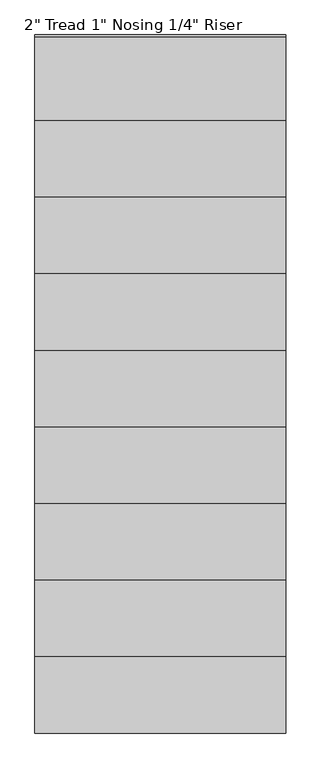
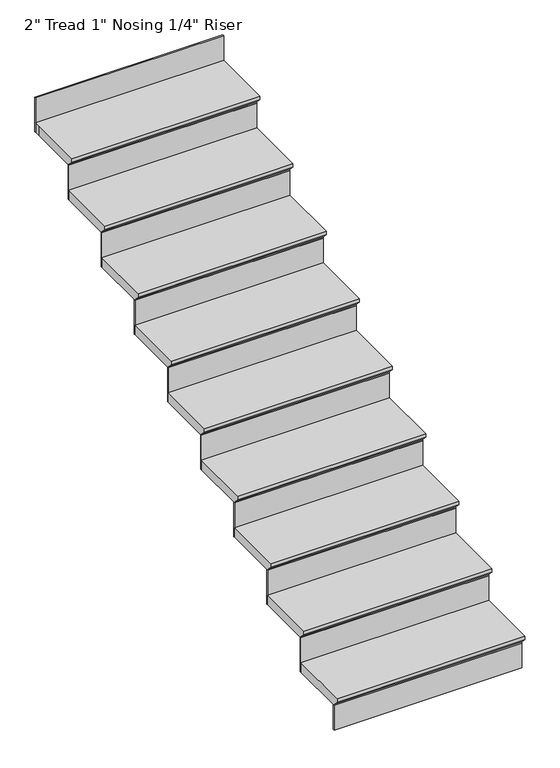
"""IFC4 building model written with IfcOpenShell, lengths in millimetres: stair flight geometry."""

from ifc_helpers import new_model, si_unit, origin, place, context, project, spatial, faceted_brep, source, transform, mapped, element, save


def stair_flight_52e4cb2b(model_context):
    return source(origin(), model_context, "Body", "Brep", [
        faceted_brep([(8378.8260838, -1689.0339187, 7169.15), (8378.8260838, -1689.0339187, 7188.2), (7464.4260838, -1689.0339187, 7188.2), (7464.4260838, -1689.0339187, 7169.15), (8378.8260838, -1663.6339187, 7143.75), (7464.4260838, -1663.6339187, 7143.75), (8378.8260838, -1384.2339187, 7188.2), (7464.4260838, -1384.2339187, 7188.2), (7464.4260838, -1663.6339187, 7137.4), (7464.4260838, -1384.2339187, 7137.4), (8378.8260838, -1384.2339187, 7137.4), (8378.8260838, -1663.6339187, 7137.4)], [[[0, 1, 2, 3]], [[4, 0, 3, 5]], [[2, 1, 6, 7]], [[8, 9, 10, 11]], [[2, 7, 9, 8, 5, 3]], [[8, 11, 4, 5]], [[6, 1, 0, 4, 11, 10]], [[7, 6, 10, 9]]]),
        faceted_brep([(8378.8260838, -1663.6339187, 7137.4), (8378.8260838, -1663.6339187, 7010.4), (8378.8260838, -1657.2839187, 7010.4), (8378.8260838, -1657.2839187, 7137.4), (7464.4260838, -1663.6339187, 7137.4), (7464.4260838, -1657.2839187, 7137.4), (7464.4260838, -1657.2839187, 7010.4), (7464.4260838, -1663.6339187, 7010.4)], [[[0, 1, 2, 3]], [[4, 5, 6, 7]], [[1, 0, 4, 7]], [[2, 1, 7, 6]], [[3, 2, 6, 5]], [[0, 3, 5, 4]]]),
        faceted_brep([(8378.8260838, -1384.2339187, 7315.2), (8378.8260838, -1384.2339187, 7137.4), (8378.8260838, -1377.8839187, 7137.4), (8378.8260838, -1377.8839187, 7315.2), (7464.4260838, -1384.2339187, 7315.2), (7464.4260838, -1377.8839187, 7315.2), (7464.4260838, -1377.8839187, 7137.4), (7464.4260838, -1384.2339187, 7137.4)], [[[0, 1, 2, 3]], [[4, 5, 6, 7]], [[1, 0, 4, 7]], [[2, 1, 7, 6]], [[3, 2, 6, 5]], [[0, 3, 5, 4]]]),
        faceted_brep([(7464.4260838, -1409.6339187, 7366.0), (8378.8260838, -1409.6339187, 7366.0), (8378.8260838, -1104.8339187, 7366.0), (7464.4260838, -1104.8339187, 7366.0), (7464.4260838, -1384.2339187, 7315.2), (7464.4260838, -1104.8339187, 7315.2), (8378.8260838, -1104.8339187, 7315.2), (8378.8260838, -1384.2339187, 7315.2), (7464.4260838, -1384.2339187, 7321.55), (7464.4260838, -1409.6339187, 7346.95), (8378.8260838, -1384.2339187, 7321.55), (8378.8260838, -1409.6339187, 7346.95)], [[[0, 1, 2, 3]], [[4, 5, 6, 7]], [[0, 3, 5, 4, 8, 9]], [[4, 7, 10, 8]], [[2, 1, 11, 10, 7, 6]], [[3, 2, 6, 5]], [[11, 1, 0, 9]], [[10, 11, 9, 8]]]),
        faceted_brep([(8378.8260838, -1104.8339187, 7493.0), (8378.8260838, -1104.8339187, 7315.2), (8378.8260838, -1098.4839187, 7315.2), (8378.8260838, -1098.4839187, 7493.0), (7464.4260838, -1104.8339187, 7493.0), (7464.4260838, -1098.4839187, 7493.0), (7464.4260838, -1098.4839187, 7315.2), (7464.4260838, -1104.8339187, 7315.2)], [[[0, 1, 2, 3]], [[4, 5, 6, 7]], [[1, 0, 4, 7]], [[2, 1, 7, 6]], [[3, 2, 6, 5]], [[0, 3, 5, 4]]]),
        faceted_brep([(7464.4260838, -1130.2339187, 7543.8), (8378.8260838, -1130.2339187, 7543.8), (8378.8260838, -825.4339187, 7543.8), (7464.4260838, -825.4339187, 7543.8), (7464.4260838, -1104.8339187, 7493.0), (7464.4260838, -825.4339187, 7493.0), (8378.8260838, -825.4339187, 7493.0), (8378.8260838, -1104.8339187, 7493.0), (7464.4260838, -1104.8339187, 7499.35), (7464.4260838, -1130.2339187, 7524.75), (8378.8260838, -1104.8339187, 7499.35), (8378.8260838, -1130.2339187, 7524.75)], [[[0, 1, 2, 3]], [[4, 5, 6, 7]], [[0, 3, 5, 4, 8, 9]], [[4, 7, 10, 8]], [[2, 1, 11, 10, 7, 6]], [[3, 2, 6, 5]], [[11, 1, 0, 9]], [[10, 11, 9, 8]]]),
        faceted_brep([(8378.8260838, -825.4339187, 7670.8), (8378.8260838, -825.4339187, 7493.0), (8378.8260838, -819.0839187, 7493.0), (8378.8260838, -819.0839187, 7670.8), (7464.4260838, -825.4339187, 7670.8), (7464.4260838, -819.0839187, 7670.8), (7464.4260838, -819.0839187, 7493.0), (7464.4260838, -825.4339187, 7493.0)], [[[0, 1, 2, 3]], [[4, 5, 6, 7]], [[1, 0, 4, 7]], [[2, 1, 7, 6]], [[3, 2, 6, 5]], [[0, 3, 5, 4]]]),
        faceted_brep([(7464.4260838, -850.8339187, 7721.6), (8378.8260838, -850.8339187, 7721.6), (8378.8260838, -546.0339187, 7721.6), (7464.4260838, -546.0339187, 7721.6), (7464.4260838, -825.4339187, 7670.8), (7464.4260838, -546.0339187, 7670.8), (8378.8260838, -546.0339187, 7670.8), (8378.8260838, -825.4339187, 7670.8), (7464.4260838, -825.4339187, 7677.15), (7464.4260838, -850.8339187, 7702.55), (8378.8260838, -825.4339187, 7677.15), (8378.8260838, -850.8339187, 7702.55)], [[[0, 1, 2, 3]], [[4, 5, 6, 7]], [[0, 3, 5, 4, 8, 9]], [[4, 7, 10, 8]], [[2, 1, 11, 10, 7, 6]], [[3, 2, 6, 5]], [[11, 1, 0, 9]], [[10, 11, 9, 8]]]),
        faceted_brep([(8378.8260838, -546.0339187, 7848.6), (8378.8260838, -546.0339187, 7670.8), (8378.8260838, -539.6839187, 7670.8), (8378.8260838, -539.6839187, 7848.6), (7464.4260838, -546.0339187, 7848.6), (7464.4260838, -539.6839187, 7848.6), (7464.4260838, -539.6839187, 7670.8), (7464.4260838, -546.0339187, 7670.8)], [[[0, 1, 2, 3]], [[4, 5, 6, 7]], [[1, 0, 4, 7]], [[2, 1, 7, 6]], [[3, 2, 6, 5]], [[0, 3, 5, 4]]]),
        faceted_brep([(7464.4260838, -571.4339187, 7899.4), (8378.8260838, -571.4339187, 7899.4), (8378.8260838, -266.6339187, 7899.4), (7464.4260838, -266.6339187, 7899.4), (7464.4260838, -546.0339187, 7848.6), (7464.4260838, -266.6339187, 7848.6), (8378.8260838, -266.6339187, 7848.6), (8378.8260838, -546.0339187, 7848.6), (7464.4260838, -546.0339187, 7854.95), (7464.4260838, -571.4339187, 7880.35), (8378.8260838, -546.0339187, 7854.95), (8378.8260838, -571.4339187, 7880.35)], [[[0, 1, 2, 3]], [[4, 5, 6, 7]], [[0, 3, 5, 4, 8, 9]], [[4, 7, 10, 8]], [[2, 1, 11, 10, 7, 6]], [[3, 2, 6, 5]], [[11, 1, 0, 9]], [[10, 11, 9, 8]]]),
        faceted_brep([(8378.8260838, -266.6339187, 8026.4), (8378.8260838, -266.6339187, 7848.6), (8378.8260838, -260.2839187, 7848.6), (8378.8260838, -260.2839187, 8026.4), (7464.4260838, -266.6339187, 8026.4), (7464.4260838, -260.2839187, 8026.4), (7464.4260838, -260.2839187, 7848.6), (7464.4260838, -266.6339187, 7848.6)], [[[0, 1, 2, 3]], [[4, 5, 6, 7]], [[1, 0, 4, 7]], [[2, 1, 7, 6]], [[3, 2, 6, 5]], [[0, 3, 5, 4]]]),
        faceted_brep([(7464.4260838, -292.0339187, 8077.2), (8378.8260838, -292.0339187, 8077.2), (8378.8260838, 12.7660813, 8077.2), (7464.4260838, 12.7660813, 8077.2), (7464.4260838, -266.6339187, 8026.4), (7464.4260838, 12.7660813, 8026.4), (8378.8260838, 12.7660813, 8026.4), (8378.8260838, -266.6339187, 8026.4), (7464.4260838, -266.6339187, 8032.75), (7464.4260838, -292.0339187, 8058.15), (8378.8260838, -266.6339187, 8032.75), (8378.8260838, -292.0339187, 8058.15)], [[[0, 1, 2, 3]], [[4, 5, 6, 7]], [[0, 3, 5, 4, 8, 9]], [[4, 7, 10, 8]], [[2, 1, 11, 10, 7, 6]], [[3, 2, 6, 5]], [[11, 1, 0, 9]], [[10, 11, 9, 8]]]),
        faceted_brep([(8378.8260838, 12.7660813, 8204.2), (8378.8260838, 12.7660813, 8026.4), (8378.8260838, 19.1160813, 8026.4), (8378.8260838, 19.1160813, 8204.2), (7464.4260838, 12.7660813, 8204.2), (7464.4260838, 19.1160813, 8204.2), (7464.4260838, 19.1160813, 8026.4), (7464.4260838, 12.7660813, 8026.4)], [[[0, 1, 2, 3]], [[4, 5, 6, 7]], [[1, 0, 4, 7]], [[2, 1, 7, 6]], [[3, 2, 6, 5]], [[0, 3, 5, 4]]]),
        faceted_brep([(7464.4260838, -12.6339187, 8255.0), (8378.8260838, -12.6339187, 8255.0), (8378.8260838, 292.1660813, 8255.0), (7464.4260838, 292.1660813, 8255.0), (7464.4260838, 12.7660813, 8204.2), (7464.4260838, 292.1660813, 8204.2), (8378.8260838, 292.1660813, 8204.2), (8378.8260838, 12.7660813, 8204.2), (7464.4260838, 12.7660813, 8210.55), (7464.4260838, -12.6339187, 8235.95), (8378.8260838, 12.7660813, 8210.55), (8378.8260838, -12.6339187, 8235.95)], [[[0, 1, 2, 3]], [[4, 5, 6, 7]], [[0, 3, 5, 4, 8, 9]], [[4, 7, 10, 8]], [[2, 1, 11, 10, 7, 6]], [[3, 2, 6, 5]], [[11, 1, 0, 9]], [[10, 11, 9, 8]]]),
        faceted_brep([(8378.8260838, 292.1660813, 8382.0), (8378.8260838, 292.1660813, 8204.2), (8378.8260838, 298.5160813, 8204.2), (8378.8260838, 298.5160813, 8382.0), (7464.4260838, 292.1660813, 8382.0), (7464.4260838, 298.5160813, 8382.0), (7464.4260838, 298.5160813, 8204.2), (7464.4260838, 292.1660813, 8204.2)], [[[0, 1, 2, 3]], [[4, 5, 6, 7]], [[1, 0, 4, 7]], [[2, 1, 7, 6]], [[3, 2, 6, 5]], [[0, 3, 5, 4]]]),
        faceted_brep([(7464.4260838, 266.7660813, 8432.8), (8378.8260838, 266.7660813, 8432.8), (8378.8260838, 571.5660813, 8432.8), (7464.4260838, 571.5660813, 8432.8), (7464.4260838, 292.1660813, 8382.0), (7464.4260838, 571.5660813, 8382.0), (8378.8260838, 571.5660813, 8382.0), (8378.8260838, 292.1660813, 8382.0), (7464.4260838, 292.1660813, 8388.35), (7464.4260838, 266.7660813, 8413.75), (8378.8260838, 292.1660813, 8388.35), (8378.8260838, 266.7660813, 8413.75)], [[[0, 1, 2, 3]], [[4, 5, 6, 7]], [[0, 3, 5, 4, 8, 9]], [[4, 7, 10, 8]], [[2, 1, 11, 10, 7, 6]], [[3, 2, 6, 5]], [[11, 1, 0, 9]], [[10, 11, 9, 8]]]),
        faceted_brep([(8378.8260838, 850.9660813, 8737.6), (8378.8260838, 850.9660813, 8559.8), (8378.8260838, 857.3160813, 8559.8), (8378.8260838, 857.3160813, 8737.6), (7464.4260838, 850.9660813, 8737.6), (7464.4260838, 857.3160813, 8737.6), (7464.4260838, 857.3160813, 8559.8), (7464.4260838, 850.9660813, 8559.8)], [[[0, 1, 2, 3]], [[4, 5, 6, 7]], [[1, 0, 4, 7]], [[2, 1, 7, 6]], [[3, 2, 6, 5]], [[0, 3, 5, 4]]]),
        faceted_brep([(8378.8260838, 571.5660813, 8559.8), (8378.8260838, 571.5660813, 8382.0), (8378.8260838, 577.9160813, 8382.0), (8378.8260838, 577.9160813, 8559.8), (7464.4260838, 571.5660813, 8559.8), (7464.4260838, 577.9160813, 8559.8), (7464.4260838, 577.9160813, 8382.0), (7464.4260838, 571.5660813, 8382.0)], [[[0, 1, 2, 3]], [[4, 5, 6, 7]], [[1, 0, 4, 7]], [[2, 1, 7, 6]], [[3, 2, 6, 5]], [[0, 3, 5, 4]]]),
        faceted_brep([(7464.4260838, 850.9660813, 8610.6), (7464.4260838, 825.5660813, 8610.6), (7464.4260838, 546.1660813, 8610.6), (8378.8260838, 546.1660813, 8610.6), (8378.8260838, 850.9660813, 8610.6), (7464.4260838, 825.5660813, 8559.8), (7464.4260838, 850.9660813, 8559.8), (8378.8260838, 850.9660813, 8559.8), (8378.8260838, 571.5660813, 8559.8), (7464.4260838, 571.5660813, 8559.8), (7464.4260838, 571.5660813, 8566.15), (7464.4260838, 546.1660813, 8591.55), (8378.8260838, 571.5660813, 8566.15), (8378.8260838, 546.1660813, 8591.55)], [[[0, 1, 2, 3, 4]], [[5, 6, 7, 8, 9]], [[1, 0, 6, 5]], [[2, 1, 5, 9, 10, 11]], [[9, 8, 12, 10]], [[4, 3, 13, 12, 8, 7]], [[0, 4, 7, 6]], [[13, 3, 2, 11]], [[12, 13, 11, 10]]]),
    ])


if __name__ == "__main__":
    model = new_model("IFC4")
    model_context = context("Model", 3, world=origin())
    ifc_project = project(units=[si_unit("LENGTHUNIT", "METRE", prefix="MILLI")], contexts=[model_context])
    site = spatial("IfcSite", under=ifc_project)
    building = spatial("IfcBuilding", under=site)
    placement = place(None, origin())
    stair_flight_shape = stair_flight_52e4cb2b(model_context)
    element("IfcStairFlight", 1, ObjectType="2\" Tread 1\" Nosing 1/4\" Riser", at=placement, inside=building, context=model_context, shape_type="MappedRepresentation", body=[
        mapped(stair_flight_shape, transform((0.0, 0.0, 0.0), x_axis=(1.0, 0.0, 0.0), y_axis=(0.0, 1.0, 0.0), z_axis=(0.0, 0.0, 1.0))),
    ])
    save(model, "model.ifc")
